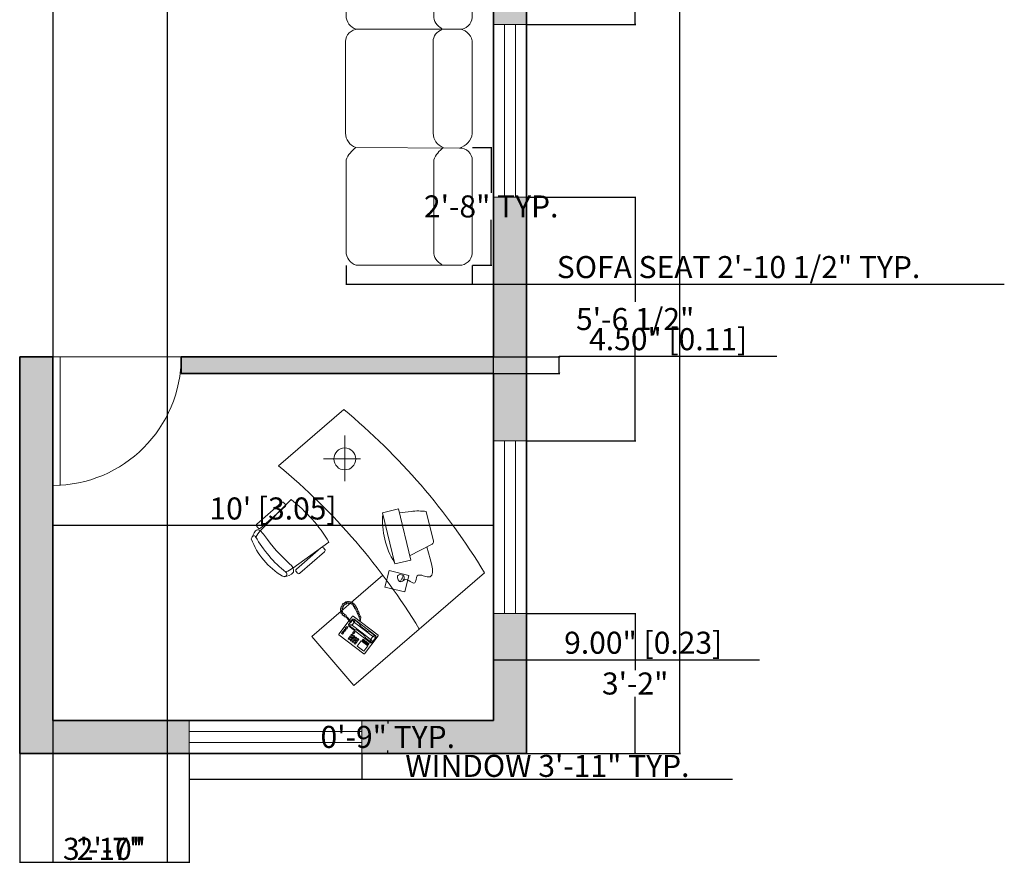
# Model space of a CAD drawing. Units: inches. Extents: x 2322 to 2932, y 142 to 762.
# Tile 2 of 7: x 2664 to 2932, y 146 to 376. Entities that reach past the tile are written whole.
import ezdxf

# ---------------------------------------------------------------- set-up
doc = ezdxf.new("R2010")
doc.units = ezdxf.units.IN
doc.header["$MEASUREMENT"] = 0
for name, color, linetype, lineweight in [('A-ANNO-DIMS', 2, 'Continuous', 18), ('A-DOOR', 3, 'Continuous', 18), ('A-EQPM', 8, 'Continuous', 15), ('A-GLAZ', 4, 'Continuous', 18), ('A-WALL', 7, 'Continuous', 35)]:
    doc.layers.add(name, color=color, linetype=linetype, lineweight=lineweight)
doc.layers.add('A-WALL-PATT', color=40, linetype='Continuous', lineweight=13, true_color=0xf8d731)
doc.layers.add('Furniture', color=7, linetype='Continuous', lineweight=15, true_color=0xffffff)
doc.styles.get("Standard").update_dxf_attribs({"font": 'italic8.shx'})
doc.dimstyles.get("Standard").update_dxf_attribs({"dimtxt": 6, "dimasz": 0.15, "dimexe": 0.18, "dimexo": 0.0625, "dimgap": 0.09, "dimtad": 1, "dimtih": 1, "dimtoh": 1, "dimzin": 0, "dimdsep": 46, "dimlunit": 3, "dimtxsty": 'Standard', "dimblk": 'CLOSEDBLANK', "dimcen": 0.09, "dimclrd": 3, "dimclre": 1, "dimclrt": 6, "dimadec": 0, "dimazin": 0, "dimtfac": 1, "dimtofl": 0, "dimtmove": 0, "dimatfit": 3, "dimldrblk": 'DOT', "dimfxl": 1, "dimtolj": 1, "dimtzin": 0, "dimarcsym": 0})

# ---------------------------------------------------------------- blocks, each defined once
blk = doc.blocks.new('_ClosedBlank')
at = {"color": 0, "linetype": 'ByBlock', "lineweight": -2}
for p, q in [((-1, 0.2), (0, 0)), ((-1, 0.2), (-1, -0.2)), ((0, 0), (-1, -0.2))]:
    blk.add_line(p, q, dxfattribs=at)
blk = doc.blocks.new('*D3')
at = {"layer": 'A-ANNO-DIMS', "color": 0, "lineweight": -2, "transparency": 16777216}
for p, q in [((2802.13, 718.82), (2844.02, 718.82)), ((2843.84, 718.67), (2843.84, 451.98)), ((2843.84, 175.97), (2843.84, 442.66)), ((2802.13, 175.82), (2844.02, 175.82))]:
    blk.add_line(p, q, dxfattribs=at)
at = {"layer": 'Defpoints', "color": 0, "transparency": 16777216}
for p in [(2802.06, 718.82), (2802.06, 175.82), (2843.84, 175.82)]:
    blk.add_point(p, dxfattribs=at)
at = {"layer": 'A-ANNO-DIMS', "color": 0, "lineweight": -2, "transparency": 16777216, "xscale": 0.15, "yscale": 0.15, "zscale": 0.15}
for p, rotation in [((2843.84, 718.82), 90), ((2843.84, 175.82), 270)]:
    blk.add_blockref('_ClosedBlank', p, dxfattribs=dict(at, rotation=rotation))
at = {"layer": 'A-ANNO-DIMS', "color": 0, "transparency": 16777216, "insert": (2843.84, 447.32), "char_height": 6, "attachment_point": 5}
blk.add_mtext('\\A1;45\'-3.00" [13.79]', dxfattribs=at)
blk = doc.blocks.new('_Dot')
at = {"color": 0, "linetype": 'ByBlock', "lineweight": -2}
blk.add_line((-0.5, 0), (-1, 0), dxfattribs=at)
at = {"color": 0, "linetype": 'ByBlock', "const_width": 0.5}
blk.add_lwpolyline([(-0.25, 0, 1), (0.25, 0, 1)], format="xyb", close=True, dxfattribs=at)
blk = doc.blocks.new('*D4')
at = {"layer": 'A-ANNO-DIMS', "color": 0, "lineweight": -2, "transparency": 16777216}
for p, q in [((2673.06, 234.35), (2673.06, 238.01)), ((2792.91, 237.83), (2673.21, 237.83)), ((2793.06, 237.77), (2793.06, 237.65))]:
    blk.add_line(p, q, dxfattribs=at)
at = {"layer": 'Defpoints', "color": 0, "transparency": 16777216}
for p in [(2673.06, 237.83), (2793.06, 237.83), (2673.06, 234.29)]:
    blk.add_point(p, dxfattribs=at)
at = {"layer": 'A-ANNO-DIMS', "color": 0, "lineweight": -2, "transparency": 16777216, "xscale": 0.15, "yscale": 0.15, "zscale": 0.15, "rotation": 180}
blk.add_blockref('_ClosedBlank', (2673.06, 237.83), dxfattribs=at)
at = {"layer": 'A-ANNO-DIMS', "color": 0, "lineweight": -2, "transparency": 16777216, "xscale": 0.15, "yscale": 0.15, "zscale": 0.15}
blk.add_blockref('_ClosedBlank', (2793.06, 237.83), dxfattribs=at)
at = {"layer": 'A-ANNO-DIMS', "color": 0, "transparency": 16777216, "insert": (2733.06, 242.49), "char_height": 6, "attachment_point": 5}
blk.add_mtext("\\A1;10' [3.05]", dxfattribs=at)
blk = doc.blocks.new('*D5')
at = {"layer": 'A-ANNO-DIMS', "color": 0, "lineweight": -2, "transparency": 16777216}
for p, q in [((2793.06, 307.6), (2793.06, 201.1)), ((2802.06, 307.6), (2802.06, 201.1)), ((2793.21, 201.28), (2801.91, 201.28)), ((2802.06, 201.28), (2865.54, 201.28))]:
    blk.add_line(p, q, dxfattribs=at)
at = {"layer": 'Defpoints', "color": 0, "transparency": 16777216}
for p in [(2793.06, 307.66), (2802.06, 307.66), (2802.06, 201.28)]:
    blk.add_point(p, dxfattribs=at)
at = {"layer": 'A-ANNO-DIMS', "color": 0, "lineweight": -2, "transparency": 16777216, "xscale": 0.15, "yscale": 0.15, "zscale": 0.15, "rotation": 180}
blk.add_blockref('_ClosedBlank', (2793.06, 201.28), dxfattribs=at)
at = {"layer": 'A-ANNO-DIMS', "color": 0, "lineweight": -2, "transparency": 16777216, "xscale": 0.15, "yscale": 0.15, "zscale": 0.15}
blk.add_blockref('_ClosedBlank', (2802.06, 201.28), dxfattribs=at)
at = {"layer": 'A-ANNO-DIMS', "color": 0, "transparency": 16777216, "insert": (2833.88, 205.95), "char_height": 6, "attachment_point": 5}
blk.add_mtext('\\A1;9.00" [0.23]', dxfattribs=at)
blk = doc.blocks.new('*D6')
at = {"layer": 'A-ANNO-DIMS', "color": 0, "lineweight": -2, "transparency": 16777216}
for p, q in [((2743.62, 283.76), (2811.19, 283.76)), ((2811.01, 283.76), (2811.01, 283.91)), ((2811.01, 283.91), (2870.24, 283.91)), ((2811.01, 279.41), (2811.01, 283.61)), ((2743.62, 279.26), (2811.19, 279.26))]:
    blk.add_line(p, q, dxfattribs=at)
at = {"layer": 'Defpoints', "color": 0, "transparency": 16777216}
for p in [(2743.55, 283.76), (2811.01, 283.76), (2743.55, 279.26)]:
    blk.add_point(p, dxfattribs=at)
at = {"layer": 'A-ANNO-DIMS', "color": 0, "lineweight": -2, "transparency": 16777216, "xscale": 0.15, "yscale": 0.15, "zscale": 0.15}
for p, rotation in [((2811.01, 283.76), 90), ((2811.01, 279.26), 270)]:
    blk.add_blockref('_ClosedBlank', p, dxfattribs=dict(at, rotation=rotation))
at = {"layer": 'A-ANNO-DIMS', "color": 0, "transparency": 16777216, "insert": (2840.67, 288.57), "char_height": 6, "attachment_point": 5}
blk.add_mtext('\\A1;4.50" [0.11]', dxfattribs=at)
blk = doc.blocks.new('DOOR-SWING-35')
for p, q in [((0, 35), (0, 0)), ((2, 35), (2, 0)), ((0, 0), (35, 0))]:
    blk.add_line(p, q)
blk.add_arc((0, 0), 35, 0, 90)
blk = doc.blocks.new('WINDOW-47X9')
for p, q in [((47, 9), (0, 9)), ((0, 9), (0, 0)), ((47, 0), (47, 9)), ((0, 6), (47, 6)), ((0, 3), (47, 3)), ((0, 0), (47, 0))]:
    blk.add_line(p, q)
blk = doc.blocks.new('SECTIONAL-SEAT')
for p, q in [((30.86, 31.9), (2.62, 32.04)), ((0, 28.69), (0, 3.79)), ((23.85, 28.69), (23.85, 3.79)), ((34.36, 3.2), (34.36, 28.55)), ((2.77, 0), (30.86, 0))]:
    blk.add_line(p, q)
for centre, radius, start, end in [((7.53, 25.51), 8.17, 126.8838, 157.0502), ((31.38, 25.51), 8.17, 126.8838, 157.0502), ((31, 28.55), 3.35, 0, 92.4088), ((3.98, 3.79), 3.98, 180, 252.2888), ((27.83, 3.79), 3.98, 180, 244.0743), ((30.86, 3.51), 3.51, 270, 355.0498)]:
    blk.add_arc(centre, radius, start, end)
blk = doc.blocks.new('*D28')
at = {"layer": 'A-ANNO-DIMS', "color": 1, "lineweight": -2, "transparency": 16777216}
for p, q in [((2710.26, 175.76), (2710.26, 168.59)), ((2757.26, 175.76), (2757.26, 168.59))]:
    blk.add_line(p, q, dxfattribs=at)
at = {"layer": 'A-ANNO-DIMS', "color": 3, "lineweight": -2, "transparency": 16777216}
for p, q in [((2710.41, 168.77), (2757.11, 168.77)), ((2757.26, 168.77), (2858.16, 168.77))]:
    blk.add_line(p, q, dxfattribs=at)
at = {"layer": 'Defpoints', "color": 0, "transparency": 16777216}
for p in [(2710.26, 175.82), (2757.26, 175.82), (2757.26, 168.77)]:
    blk.add_point(p, dxfattribs=at)
at = {"layer": 'A-ANNO-DIMS', "color": 3, "lineweight": -2, "transparency": 16777216, "xscale": 0.15, "yscale": 0.15, "zscale": 0.15, "rotation": 180}
blk.add_blockref('_ClosedBlank', (2710.26, 168.77), dxfattribs=at)
at = {"layer": 'A-ANNO-DIMS', "color": 3, "lineweight": -2, "transparency": 16777216, "xscale": 0.15, "yscale": 0.15, "zscale": 0.15}
blk.add_blockref('_ClosedBlank', (2757.26, 168.77), dxfattribs=at)
at = {"layer": 'A-ANNO-DIMS', "color": 6, "transparency": 16777216, "insert": (2807.78, 172.43), "char_height": 6, "attachment_point": 5}
blk.add_mtext('\\A1;WINDOW 3\'-11" TYP.', dxfattribs=at)
blk = doc.blocks.new('*D29')
at = {"layer": 'A-ANNO-DIMS', "color": 1, "lineweight": -2, "transparency": 16777216}
for p, q in [((2757.32, 184.82), (2764.49, 184.82)), ((2757.32, 175.82), (2764.49, 175.82))]:
    blk.add_line(p, q, dxfattribs=at)
at = {"layer": 'A-ANNO-DIMS', "color": 3, "lineweight": -2, "transparency": 16777216}
for p, q in [((2764.31, 184.67), (2764.31, 183.98)), ((2764.31, 175.97), (2764.31, 176.66))]:
    blk.add_line(p, q, dxfattribs=at)
at = {"layer": 'Defpoints', "color": 0, "transparency": 16777216}
for p in [(2757.26, 184.82), (2764.31, 184.82), (2757.26, 175.82)]:
    blk.add_point(p, dxfattribs=at)
at = {"layer": 'A-ANNO-DIMS', "color": 3, "lineweight": -2, "transparency": 16777216, "xscale": 0.15, "yscale": 0.15, "zscale": 0.15}
for p, rotation in [((2764.31, 184.82), 90), ((2764.31, 175.82), 270)]:
    blk.add_blockref('_ClosedBlank', p, dxfattribs=dict(at, rotation=rotation))
at = {"layer": 'A-ANNO-DIMS', "color": 6, "transparency": 16777216, "insert": (2764.31, 180.32), "char_height": 6, "attachment_point": 5}
blk.add_mtext('\\A1;0\'-9" TYP.', dxfattribs=at)
blk = doc.blocks.new('*D40')
at = {"layer": 'A-ANNO-DIMS', "color": 1, "lineweight": -2, "transparency": 16777216}
for p, q in [((2752.97, 308.61), (2752.97, 303.34)), ((2787.33, 308.61), (2787.33, 303.34))]:
    blk.add_line(p, q, dxfattribs=at)
at = {"layer": 'A-ANNO-DIMS', "color": 3, "lineweight": -2, "transparency": 16777216}
for p, q in [((2753.12, 303.52), (2787.18, 303.52)), ((2787.33, 303.52), (2932.23, 303.52))]:
    blk.add_line(p, q, dxfattribs=at)
at = {"layer": 'Defpoints', "color": 0, "transparency": 16777216}
for p in [(2752.97, 308.68), (2787.33, 308.68), (2787.33, 303.52)]:
    blk.add_point(p, dxfattribs=at)
at = {"layer": 'A-ANNO-DIMS', "color": 3, "lineweight": -2, "transparency": 16777216, "xscale": 0.15, "yscale": 0.15, "zscale": 0.15, "rotation": 180}
blk.add_blockref('_ClosedBlank', (2752.97, 303.52), dxfattribs=at)
at = {"layer": 'A-ANNO-DIMS', "color": 3, "lineweight": -2, "transparency": 16777216, "xscale": 0.15, "yscale": 0.15, "zscale": 0.15}
blk.add_blockref('_ClosedBlank', (2787.33, 303.52), dxfattribs=at)
at = {"layer": 'A-ANNO-DIMS', "color": 6, "transparency": 16777216, "insert": (2859.85, 308.19), "char_height": 6, "attachment_point": 5}
blk.add_mtext('\\A1;SOFA SEAT 2\'-10 1/2" TYP.', dxfattribs=at)
blk = doc.blocks.new('*D41')
at = {"layer": 'A-ANNO-DIMS', "color": 1, "lineweight": -2, "transparency": 16777216}
for p, q in [((2787.39, 340.72), (2792.66, 340.72)), ((2787.39, 308.68), (2792.66, 308.68))]:
    blk.add_line(p, q, dxfattribs=at)
at = {"layer": 'A-ANNO-DIMS', "color": 3, "lineweight": -2, "transparency": 16777216}
for p, q in [((2792.48, 340.57), (2792.48, 328.36)), ((2792.48, 308.83), (2792.48, 321.04))]:
    blk.add_line(p, q, dxfattribs=at)
at = {"layer": 'Defpoints', "color": 0, "transparency": 16777216}
for p in [(2787.33, 340.72), (2792.48, 340.72), (2787.33, 308.68)]:
    blk.add_point(p, dxfattribs=at)
at = {"layer": 'A-ANNO-DIMS', "color": 3, "lineweight": -2, "transparency": 16777216, "xscale": 0.15, "yscale": 0.15, "zscale": 0.15}
for p, rotation in [((2792.48, 340.72), 90), ((2792.48, 308.68), 270)]:
    blk.add_blockref('_ClosedBlank', p, dxfattribs=dict(at, rotation=rotation))
at = {"layer": 'A-ANNO-DIMS', "color": 6, "transparency": 16777216, "insert": (2792.48, 324.7), "char_height": 6, "attachment_point": 5}
blk.add_mtext('\\A1;2\'-8" TYP.', dxfattribs=at)
blk = doc.blocks.new('*D54')
at = {"layer": 'A-ANNO-DIMS', "color": 1, "lineweight": -2, "transparency": 16777216}
for p, q in [((2673.06, 709.76), (2673.06, 146.01)), ((2704.23, 709.76), (2704.23, 146.01))]:
    blk.add_line(p, q, dxfattribs=at)
at = {"layer": 'A-ANNO-DIMS', "color": 3, "lineweight": -2, "transparency": 16777216}
blk.add_line((2673.21, 146.19), (2704.08, 146.19), dxfattribs=at)
at = {"layer": 'Defpoints', "color": 0, "transparency": 16777216}
for p in [(2673.06, 709.82), (2704.23, 709.82), (2704.23, 146.19)]:
    blk.add_point(p, dxfattribs=at)
at = {"layer": 'A-ANNO-DIMS', "color": 3, "lineweight": -2, "transparency": 16777216, "xscale": 0.15, "yscale": 0.15, "zscale": 0.15, "rotation": 180}
blk.add_blockref('_ClosedBlank', (2673.06, 146.19), dxfattribs=at)
at = {"layer": 'A-ANNO-DIMS', "color": 3, "lineweight": -2, "transparency": 16777216, "xscale": 0.15, "yscale": 0.15, "zscale": 0.15}
blk.add_blockref('_ClosedBlank', (2704.23, 146.19), dxfattribs=at)
at = {"layer": 'A-ANNO-DIMS', "color": 6, "transparency": 16777216, "insert": (2688.65, 149.85), "char_height": 6, "attachment_point": 5}
blk.add_mtext('\\A1;2\'-7"', dxfattribs=at)
blk = doc.blocks.new('*D61')
at = {"layer": 'A-ANNO-DIMS', "color": 1, "lineweight": -2, "transparency": 16777216}
for p, q in [((2802.13, 213.88), (2831.87, 213.88)), ((2802.13, 175.82), (2831.87, 175.82))]:
    blk.add_line(p, q, dxfattribs=at)
at = {"layer": 'A-ANNO-DIMS', "color": 3, "lineweight": -2, "transparency": 16777216}
for p, q in [((2831.69, 213.73), (2831.69, 198.51)), ((2831.69, 175.97), (2831.69, 191.19))]:
    blk.add_line(p, q, dxfattribs=at)
at = {"layer": 'Defpoints', "color": 0, "transparency": 16777216}
for p in [(2802.06, 213.88), (2831.69, 213.88), (2802.06, 175.82)]:
    blk.add_point(p, dxfattribs=at)
at = {"layer": 'A-ANNO-DIMS', "color": 3, "lineweight": -2, "transparency": 16777216, "xscale": 0.15, "yscale": 0.15, "zscale": 0.15}
for p, rotation in [((2831.69, 213.88), 90), ((2831.69, 175.82), 270)]:
    blk.add_blockref('_ClosedBlank', p, dxfattribs=dict(at, rotation=rotation))
at = {"layer": 'A-ANNO-DIMS', "color": 6, "transparency": 16777216, "insert": (2831.69, 194.85), "char_height": 6, "attachment_point": 5}
blk.add_mtext('\\A1;3\'-2"', dxfattribs=at)
blk = doc.blocks.new('*D62')
at = {"layer": 'A-ANNO-DIMS', "color": 1, "lineweight": -2, "transparency": 16777216}
for p, q in [((2802.13, 327.22), (2831.87, 327.22)), ((2802.13, 260.88), (2831.87, 260.88))]:
    blk.add_line(p, q, dxfattribs=at)
at = {"layer": 'A-ANNO-DIMS', "color": 3, "lineweight": -2, "transparency": 16777216}
for p, q in [((2831.69, 327.07), (2831.69, 298.71)), ((2831.69, 261.03), (2831.69, 289.39))]:
    blk.add_line(p, q, dxfattribs=at)
at = {"layer": 'Defpoints', "color": 0, "transparency": 16777216}
for p in [(2802.06, 327.22), (2831.69, 327.22), (2802.06, 260.88)]:
    blk.add_point(p, dxfattribs=at)
at = {"layer": 'A-ANNO-DIMS', "color": 3, "lineweight": -2, "transparency": 16777216, "xscale": 0.15, "yscale": 0.15, "zscale": 0.15}
for p, rotation in [((2831.69, 327.22), 90), ((2831.69, 260.88), 270)]:
    blk.add_blockref('_ClosedBlank', p, dxfattribs=dict(at, rotation=rotation))
at = {"layer": 'A-ANNO-DIMS', "color": 6, "transparency": 16777216, "insert": (2831.69, 294.05), "char_height": 6, "attachment_point": 5}
blk.add_mtext('\\A1;5\'-6 1/2"', dxfattribs=at)
blk = doc.blocks.new('*D63')
at = {"layer": 'A-ANNO-DIMS', "color": 1, "lineweight": -2, "transparency": 16777216}
for p, q in [((2802.13, 431.57), (2831.87, 431.57)), ((2802.13, 374.22), (2831.87, 374.22))]:
    blk.add_line(p, q, dxfattribs=at)
at = {"layer": 'A-ANNO-DIMS', "color": 3, "lineweight": -2, "transparency": 16777216}
for p, q in [((2831.69, 431.42), (2831.69, 407.55)), ((2831.69, 374.37), (2831.69, 398.23))]:
    blk.add_line(p, q, dxfattribs=at)
at = {"layer": 'Defpoints', "color": 0, "transparency": 16777216}
for p in [(2802.06, 431.57), (2831.69, 431.57), (2802.06, 374.22)]:
    blk.add_point(p, dxfattribs=at)
at = {"layer": 'A-ANNO-DIMS', "color": 3, "lineweight": -2, "transparency": 16777216, "xscale": 0.15, "yscale": 0.15, "zscale": 0.15}
for p, rotation in [((2831.69, 431.57), 90), ((2831.69, 374.22), 270)]:
    blk.add_blockref('_ClosedBlank', p, dxfattribs=dict(at, rotation=rotation))
at = {"layer": 'A-ANNO-DIMS', "color": 6, "transparency": 16777216, "insert": (2831.69, 402.89), "char_height": 6, "attachment_point": 5}
blk.add_mtext('\\A1;4\'-9 1/2"', dxfattribs=at)
blk = doc.blocks.new('*D65')
at = {"layer": 'A-ANNO-DIMS', "color": 1, "lineweight": -2, "transparency": 16777216}
for p, q in [((2664.06, 175.76), (2664.06, 146.01)), ((2710.26, 175.76), (2710.26, 146.01))]:
    blk.add_line(p, q, dxfattribs=at)
at = {"layer": 'A-ANNO-DIMS', "color": 3, "lineweight": -2, "transparency": 16777216}
blk.add_line((2664.21, 146.19), (2710.11, 146.19), dxfattribs=at)
at = {"layer": 'Defpoints', "color": 0, "transparency": 16777216}
for p in [(2664.06, 175.82), (2710.26, 175.82), (2710.26, 146.19)]:
    blk.add_point(p, dxfattribs=at)
at = {"layer": 'A-ANNO-DIMS', "color": 3, "lineweight": -2, "transparency": 16777216, "xscale": 0.15, "yscale": 0.15, "zscale": 0.15, "rotation": 180}
blk.add_blockref('_ClosedBlank', (2664.06, 146.19), dxfattribs=at)
at = {"layer": 'A-ANNO-DIMS', "color": 3, "lineweight": -2, "transparency": 16777216, "xscale": 0.15, "yscale": 0.15, "zscale": 0.15}
blk.add_blockref('_ClosedBlank', (2710.26, 146.19), dxfattribs=at)
at = {"layer": 'A-ANNO-DIMS', "color": 6, "transparency": 16777216, "insert": (2687.16, 149.85), "char_height": 6, "attachment_point": 5}
blk.add_mtext('\\A1;3\'-10"', dxfattribs=at)

msp = doc.modelspace()

# ---------------------------------------------------------------- hatches: boundary and pattern name
at = {"layer": 'A-WALL-PATT'}
h = msp.add_hatch(color=256, dxfattribs=at)
h.dxf.hatch_style = 1
h.paths.add_polyline_path([(2559.693, 283.756), (2439.065, 283.756), (2439.065, 295.453), (2430.065, 295.453), (2430.065, 274.756), (2559.693, 274.756)])
h.paths.add_polyline_path([(2802.065, 431.568), (2793.065, 431.568), (2793.065, 374.218), (2802.065, 374.218)])
h.paths.add_polyline_path([(2802.065, 327.218), (2793.065, 327.218), (2793.065, 283.756), (2708.065, 283.756), (2708.065, 279.256), (2793.065, 279.256), (2793.065, 260.879), (2802.065, 260.879)])
h.paths.add_polyline_path([(2673.065, 283.756), (2664.065, 283.756), (2664.065, 175.819), (2710.255, 175.819), (2710.255, 184.819), (2673.065, 184.819)])
h.paths.add_polyline_path([(2802.065, 213.879), (2793.065, 213.879), (2793.065, 184.819), (2757.255, 184.819), (2757.255, 175.819), (2802.065, 175.819)])

# ---------------------------------------------------------------- linework, layer by layer
at = {"layer": 'A-EQPM'}
for p, q in [((2767.2, 242.392), (2762.863, 241.346)), ((2770.565, 228.443), (2767.2, 242.392)), ((2767.439, 241.306), (2770.668, 241.706)), ((2776.743, 233.57), (2774.796, 241.654)), ((2762.863, 241.346), (2766.228, 227.397)), ((2770.276, 229.637), (2776.445, 232.795)), ((2766.228, 227.397), (2770.565, 228.443)), ((2763.556, 221.103), (2764.685, 225.623)), ((2764.685, 225.623), (2770.048, 224.284)), ((2767.727, 222.541), (2768.488, 224.187)), ((2768.767, 223.098), (2768.158, 223.402)), ((2770.048, 224.284), (2768.919, 219.764)), ((2768.919, 219.764), (2763.556, 221.103)), ((2751.408, 214.719), (2751.752, 214.818)), ((2751.473, 214.432), (2751.408, 214.719)), ((2751.453, 214.984), (2751.477, 215.264)), ((2751.752, 214.818), (2751.453, 214.984)), ((2751.477, 215.264), (2751.859, 215.351)), ((2751.507, 215.573), (2751.607, 215.827)), ((2751.859, 215.351), (2751.507, 215.573)), ((2751.607, 215.827), (2751.975, 215.752)), ((2751.797, 216.076), (2751.907, 216.261)), ((2751.975, 215.752), (2751.797, 216.076)), ((2751.907, 216.261), (2752.249, 216.11)), ((2752.046, 215.555), (2751.923, 214.814)), ((2751.923, 214.814), (2752.112, 214.071)), ((2752.013, 216.463), (2752.208, 216.614)), ((2752.249, 216.11), (2752.013, 216.463)), ((2752.453, 216.191), (2752.046, 215.555)), ((2752.208, 216.614), (2752.484, 216.419)), ((2753.143, 216.579), (2752.453, 216.191)), ((2752.46, 216.8), (2752.661, 216.899)), ((2752.484, 216.419), (2752.46, 216.8)), ((2752.661, 216.899), (2752.938, 216.641)), ((2752.838, 217.048), (2753.099, 217.101)), ((2752.938, 216.641), (2752.838, 217.048)), ((2753.099, 217.101), (2753.277, 216.776)), ((2753.906, 216.69), (2753.143, 216.579)), ((2753.277, 216.776), (2753.37, 217.146)), ((2753.37, 217.146), (2753.589, 217.184)), ((2753.589, 217.184), (2753.751, 216.839)), ((2753.751, 216.839), (2753.882, 217.197)), ((2753.882, 217.197), (2754.142, 217.124)), ((2754.76, 216.259), (2753.906, 216.69)), ((2754.142, 217.124), (2754.229, 216.68)), ((2754.229, 216.68), (2754.455, 216.996)), ((2754.455, 216.996), (2754.685, 216.884)), ((2754.685, 216.884), (2754.636, 216.511)), ((2754.636, 216.511), (2754.962, 216.751)), ((2755.446, 215.216), (2754.76, 216.259)), ((2754.962, 216.751), (2755.173, 216.511)), ((2755.173, 216.511), (2754.968, 216.242)), ((2754.968, 216.242), (2755.327, 216.3)), ((2755.503, 216.055), (2755.25, 215.744)), ((2755.25, 215.744), (2755.58, 215.949)), ((2755.327, 216.3), (2755.503, 216.055)), ((2755.781, 214.456), (2755.446, 215.216)), ((2755.81, 215.631), (2755.552, 215.355)), ((2755.552, 215.355), (2755.978, 215.314)), ((2755.58, 215.949), (2755.81, 215.631)), ((2756.054, 215.083), (2755.762, 214.864)), ((2755.762, 214.864), (2756.145, 214.809)), ((2756.271, 214.539), (2755.976, 214.339)), ((2755.978, 215.314), (2756.054, 215.083)), ((2756.145, 214.809), (2756.271, 214.539)), ((2753.786, 211.958), (2750.971, 208.269)), ((2751.859, 214.359), (2751.473, 214.432)), ((2751.571, 214.105), (2751.859, 214.359)), ((2751.702, 213.801), (2751.571, 214.105)), ((2752.134, 213.913), (2751.702, 213.801)), ((2751.92, 213.571), (2752.134, 213.913)), ((2752.174, 213.346), (2751.92, 213.571)), ((2752.112, 214.071), (2752.702, 213.542)), ((2752.557, 213.495), (2752.174, 213.346)), ((2752.386, 213.168), (2752.557, 213.495)), ((2752.64, 213.006), (2752.386, 213.168)), ((2752.834, 213.032), (2752.64, 213.006)), ((2752.702, 213.542), (2752.962, 213.407)), ((2752.871, 212.956), (2752.834, 213.032)), ((2753.138, 212.769), (2752.871, 212.956)), ((2752.962, 213.407), (2752.955, 213.129)), ((2752.955, 213.129), (2753.222, 212.941)), ((2753.515, 212.292), (2753.138, 212.769)), ((2753.222, 212.941), (2753.438, 212.728)), ((2753.438, 212.728), (2753.815, 212.251)), ((2753.922, 211.792), (2753.515, 212.292)), ((2753.815, 212.251), (2754.081, 211.938)), ((2754.727, 213.192), (2753.918, 212.131)), ((2754.081, 211.938), (2754.454, 211.609)), ((2754.708, 212.35), (2754.268, 211.773)), ((2754.315, 211.732), (2754.682, 212.214)), ((2754.682, 212.214), (2754.931, 212.335)), ((2755.134, 211.479), (2754.682, 212.214)), ((2755.191, 212.37), (2754.708, 212.35)), ((2754.901, 213.215), (2754.727, 213.192)), ((2761.694, 208.032), (2754.901, 213.215)), ((2754.931, 212.335), (2755.165, 212.234)), ((2755.165, 212.234), (2755.27, 211.453)), ((2755.165, 212.234), (2756.494, 211.22)), ((2761.098, 207.864), (2755.191, 212.37)), ((2755.884, 214.425), (2755.781, 214.456)), ((2755.85, 214.34), (2755.884, 214.425)), ((2756.099, 213.819), (2755.85, 214.34)), ((2755.976, 214.339), (2756.342, 214.343)), ((2756.395, 213.089), (2756.099, 213.819)), ((2756.485, 214.076), (2756.16, 213.898)), ((2756.16, 213.898), (2756.549, 213.933)), ((2756.648, 213.731), (2756.338, 213.511)), ((2756.338, 213.511), (2756.748, 213.45)), ((2756.342, 214.343), (2756.485, 214.076)), ((2756.557, 212.682), (2756.395, 213.089)), ((2756.549, 213.933), (2756.648, 213.731)), ((2756.748, 212.725), (2756.557, 212.682)), ((2756.837, 213.256), (2756.56, 213.058)), ((2756.56, 213.058), (2756.941, 213.019)), ((2756.575, 211.938), (2756.673, 212.152)), ((2756.672, 212.626), (2756.748, 212.725)), ((2756.686, 212.52), (2756.672, 212.626)), ((2756.673, 212.152), (2756.677, 212.322)), ((2756.677, 212.322), (2756.686, 212.52)), ((2756.901, 212.12), (2756.722, 211.825)), ((2756.748, 213.45), (2756.837, 213.256)), ((2756.966, 212.764), (2756.839, 212.577)), ((2756.839, 212.577), (2756.922, 212.293)), ((2756.922, 212.293), (2756.901, 212.12)), ((2756.941, 213.019), (2757.02, 212.896)), ((2757.02, 212.896), (2756.966, 212.764)), ((2752.217, 209.187), (2752.593, 209.68)), ((2752.513, 208.962), (2752.217, 209.187)), ((2752.888, 209.454), (2752.513, 208.962)), ((2752.593, 209.68), (2752.888, 209.454)), ((2752.743, 209.876), (2753.119, 210.369)), ((2753.039, 209.651), (2752.743, 209.876)), ((2753.414, 210.143), (2753.039, 209.651)), ((2753.119, 210.369), (2753.414, 210.143)), ((2754.147, 211.614), (2753.619, 210.922)), ((2753.619, 210.922), (2753.677, 210.488)), ((2753.677, 210.488), (2759.634, 205.944)), ((2753.781, 211.032), (2753.729, 210.76)), ((2753.729, 210.76), (2753.888, 210.561)), ((2753.781, 211.032), (2754.196, 211.576)), ((2754.608, 210.79), (2753.781, 211.032)), ((2753.888, 210.561), (2754.669, 210.666)), ((2753.888, 210.561), (2755.217, 209.547)), ((2754.341, 211.461), (2753.922, 211.792)), ((2754.454, 211.609), (2754.341, 211.461)), ((2755.134, 211.479), (2754.608, 210.79)), ((2754.669, 210.666), (2754.608, 210.79)), ((2757.328, 208.638), (2754.669, 210.666)), ((2755.27, 211.453), (2755.134, 211.479)), ((2755.217, 209.547), (2755.539, 209.457)), ((2757.929, 209.425), (2755.27, 211.453)), ((2755.539, 209.457), (2755.897, 209.417)), ((2755.897, 209.417), (2756.28, 209.203)), ((2756.28, 209.203), (2757.215, 208.49)), ((2756.494, 211.22), (2756.665, 210.934)), ((2756.665, 210.934), (2756.799, 210.599)), ((2756.799, 210.599), (2757.106, 210.286)), ((2757.106, 210.286), (2758.041, 209.573)), ((2757.929, 209.425), (2760.144, 207.735)), ((2758.533, 209.197), (2758.041, 209.573)), ((2758.916, 208.984), (2758.533, 209.197)), ((2750.971, 208.269), (2750.995, 208.095)), ((2750.995, 208.095), (2757.788, 202.912)), ((2751.692, 208.498), (2752.067, 208.99)), ((2751.987, 208.273), (2751.692, 208.498)), ((2752.363, 208.765), (2751.987, 208.273)), ((2752.067, 208.99), (2752.363, 208.765)), ((2753.75, 207.317), (2753.525, 207.022)), ((2753.525, 207.022), (2753.82, 206.796)), ((2754.045, 207.092), (2753.75, 207.317)), ((2753.82, 206.796), (2754.045, 207.092)), ((2754.126, 207.809), (2753.9, 207.514)), ((2753.9, 207.514), (2754.196, 207.289)), ((2754.292, 206.904), (2754.066, 206.609)), ((2754.066, 206.609), (2754.362, 206.383)), ((2754.421, 207.584), (2754.126, 207.809)), ((2754.196, 207.289), (2754.421, 207.584)), ((2754.501, 208.302), (2754.276, 208.006)), ((2754.276, 208.006), (2754.571, 207.781)), ((2754.587, 206.679), (2754.292, 206.904)), ((2754.362, 206.383), (2754.587, 206.679)), ((2754.667, 207.396), (2754.442, 207.101)), ((2754.442, 207.101), (2754.737, 206.875)), ((2754.797, 208.076), (2754.501, 208.302)), ((2754.571, 207.781), (2754.797, 208.076)), ((2754.833, 206.491), (2754.608, 206.195)), ((2754.963, 207.171), (2754.667, 207.396)), ((2755.027, 208.991), (2754.727, 208.597)), ((2754.727, 208.597), (2755.022, 208.372)), ((2754.737, 206.875), (2754.963, 207.171)), ((2755.043, 207.888), (2754.817, 207.593)), ((2754.817, 207.593), (2755.113, 207.368)), ((2755.128, 206.265), (2754.833, 206.491)), ((2755.209, 206.983), (2754.983, 206.688)), ((2754.983, 206.688), (2755.279, 206.462)), ((2755.022, 208.372), (2755.322, 208.765)), ((2755.322, 208.765), (2755.027, 208.991)), ((2755.338, 207.663), (2755.043, 207.888)), ((2755.113, 207.368), (2755.338, 207.663)), ((2755.504, 206.758), (2755.209, 206.983)), ((2755.279, 206.462), (2755.504, 206.758)), ((2755.584, 207.475), (2755.359, 207.18)), ((2755.359, 207.18), (2755.654, 206.955)), ((2755.75, 206.57), (2755.525, 206.275)), ((2755.88, 207.25), (2755.584, 207.475)), ((2755.654, 206.955), (2755.88, 207.25)), ((2756.046, 206.345), (2755.75, 206.57)), ((2756.126, 207.062), (2755.9, 206.767)), ((2755.9, 206.767), (2756.196, 206.542)), ((2756.421, 206.837), (2756.126, 207.062)), ((2756.196, 206.542), (2756.421, 206.837)), ((2757.707, 208.114), (2757.215, 208.49)), ((2757.298, 206.557), (2757.599, 206.951)), ((2757.446, 206.445), (2757.298, 206.557)), ((2757.328, 208.638), (2759.543, 206.947)), ((2757.746, 206.838), (2757.446, 206.445)), ((2757.594, 206.332), (2757.894, 206.726)), ((2757.599, 206.951), (2757.746, 206.838)), ((2758.014, 207.802), (2757.707, 208.114)), ((2758.042, 206.613), (2757.741, 206.219)), ((2757.889, 206.107), (2758.189, 206.5)), ((2757.894, 206.726), (2758.042, 206.613)), ((2757.962, 202.936), (2761.718, 207.858)), ((2758.148, 207.467), (2758.014, 207.802)), ((2758.319, 207.18), (2758.148, 207.467)), ((2758.189, 206.5), (2758.337, 206.388)), ((2759.648, 206.166), (2758.319, 207.18)), ((2759.274, 208.944), (2758.916, 208.984)), ((2759.596, 208.854), (2759.274, 208.944)), ((2759.543, 206.947), (2759.679, 206.922)), ((2759.648, 206.166), (2759.543, 206.947)), ((2760.925, 207.84), (2759.596, 208.854)), ((2760.205, 207.611), (2759.679, 206.922)), ((2759.679, 206.922), (2760.131, 206.187)), ((2760.03, 205.953), (2761.157, 207.43)), ((2760.131, 206.187), (2761.032, 207.369)), ((2760.925, 207.84), (2760.144, 207.735)), ((2760.144, 207.735), (2760.205, 207.611)), ((2760.205, 207.611), (2761.032, 207.369)), ((2761.084, 207.641), (2760.925, 207.84)), ((2761.032, 207.369), (2761.084, 207.641)), ((2761.157, 207.43), (2761.098, 207.864)), ((2761.718, 207.858), (2761.694, 208.032)), ((2754.608, 206.195), (2754.903, 205.97)), ((2754.903, 205.97), (2755.128, 206.265)), ((2755.375, 206.078), (2755.149, 205.782)), ((2755.149, 205.782), (2755.445, 205.557)), ((2755.67, 205.852), (2755.375, 206.078)), ((2755.445, 205.557), (2755.67, 205.852)), ((2755.525, 206.275), (2755.82, 206.049)), ((2755.82, 206.049), (2756.046, 206.345)), ((2757.087, 206.485), (2755.998, 205.057)), ((2755.998, 205.057), (2757.819, 203.667)), ((2758.908, 205.095), (2757.087, 206.485)), ((2757.741, 206.219), (2757.594, 206.332)), ((2757.819, 203.667), (2758.908, 205.095)), ((2758.037, 205.994), (2757.889, 206.107)), ((2758.337, 206.388), (2758.037, 205.994)), ((2758.184, 205.881), (2758.485, 206.275)), ((2758.332, 205.769), (2758.184, 205.881)), ((2758.632, 206.162), (2758.332, 205.769)), ((2758.48, 205.656), (2758.78, 206.05)), ((2758.627, 205.543), (2758.48, 205.656)), ((2758.485, 206.275), (2758.632, 206.162)), ((2758.928, 205.937), (2758.627, 205.543)), ((2758.775, 205.43), (2759.075, 205.824)), ((2758.923, 205.318), (2758.775, 205.43)), ((2758.78, 206.05), (2758.928, 205.937)), ((2759.223, 205.712), (2758.923, 205.318)), ((2759.075, 205.824), (2759.223, 205.712)), ((2759.634, 205.944), (2760.03, 205.953)), ((2759.882, 206.065), (2759.648, 206.166)), ((2760.131, 206.187), (2759.882, 206.065)), ((2757.788, 202.912), (2757.962, 202.936))]:
    msp.add_line(p, q, dxfattribs=at)
for centre, radius, start, end in [((2772.523, 225.292), 16.519, 82.09319, 96.44928), ((2784.163, 239.103), 21.275, 175.10041, 212.02115), ((2776.034, 233.399), 0.73, 304.29227, 13.58257)]:
    msp.add_arc(centre, radius, start, end, dxfattribs=at)
msp.add_open_spline([(2774.912, 232.01), (2776.281, 227.665), (2778.102, 221.884), (2771.879, 225.282), (2772.126, 220.752), (2769.236, 224.056), (2767.76, 221.798), (2766.16, 224.453), (2768.832, 224.658), (2768.805, 223.513), (2768.792, 222.946)], degree=3, knots=[0, 0, 0, 0, 8.1529356, 10.8465665, 12.8708985, 15.8281788, 16.9321938, 18.8001086, 20.2650719, 21.7019675, 21.7019675, 21.7019675, 21.7019675], dxfattribs=at)
at = {"layer": 'A-WALL'}
for p, q in [((2802.065, 175.819), (2802.065, 718.819)), ((2793.065, 283.756), (2793.065, 709.819)), ((2664.065, 175.819), (2664.065, 283.756)), ((2664.065, 283.756), (2673.065, 283.756)), ((2673.065, 184.819), (2673.065, 283.756)), ((2708.065, 283.756), (2793.065, 283.756)), ((2708.065, 279.256), (2708.065, 283.756)), ((2708.065, 279.256), (2793.065, 279.256)), ((2793.065, 184.819), (2793.065, 279.256)), ((2793.065, 184.819), (2673.065, 184.819)), ((2802.065, 175.819), (2664.065, 175.819))]:
    msp.add_line(p, q, dxfattribs=at)
at = {"layer": 'Furniture'}
for p, q in [((2784.126, 372.91), (2756.175, 372.91)), ((2752.826, 369.56), (2752.826, 350.917)), ((2776.677, 369.56), (2776.677, 350.917)), ((2787.329, 344.508), (2787.329, 369.123)), ((2752.826, 350.917), (2752.826, 344.654)), ((2776.677, 350.917), (2776.677, 344.654)), ((2734.569, 254.105, -13.399), (2752.346, 269.429, -13.399)), ((2752.6, 249.878), (2752.6, 262.374)), ((2756.919, 255.977), (2746.791, 255.977)), ((2735.391, 244.1), (2728.683, 238.239)), ((2737.987, 244.903), (2729.67, 236.477)), ((2736.403, 243.644), (2736.043, 244.056)), ((2729.651, 237.132), (2736.359, 242.992)), ((2728.639, 237.588), (2728.999, 237.176)), ((2738.461, 226.275), (2748.275, 233.29)), ((2746.126, 231.811), (2739.418, 225.951)), ((2740.386, 224.844), (2747.094, 230.704)), ((2747.138, 231.356), (2746.778, 231.767)), ((2739.374, 225.299), (2739.734, 224.888)), ((2743.61, 207.67, -13.399), (2762.955, 224.346, -13.399)), ((2790.658, 224.986, -13.399), (2772.881, 209.661, -13.399)), ((2772.881, 209.661, -13.399), (2755.103, 194.337, -13.399)), ((2755.103, 194.337, -13.399), (2743.61, 207.67, -13.399))]:
    msp.add_line(p, q, dxfattribs=at)
msp.add_circle((2752.6, 255.977), 2.981, dxfattribs=at)
for centre, radius, start, end in [((2756.175, 369.562), 3.348, 90, 180.02896), ((2780.025, 369.562), 3.348, 106.75774, 180.02896), ((2783.489, 369.123), 3.84, 0, 80.44416), ((2757.005, 344.654), 4.179, 180, 250.24112), ((2780.856, 344.654), 4.179, 180, 250.24112), ((2782.449, 345.325), 4.948, 286.26799, 350.49369), ((2640.011, 133.858, -13.399), 176.065, 31.17046, 50.35492), ((2622.234, 118.533, -13.399), 176.065, 31.17046, 50.35492), ((2735.695, 243.752), 0.462, 41.14063, 131.14063), ((2713.514, 212.856), 40.322, 30.44798, 52.63235), ((2736.055, 243.34), 0.462, 311.14063, 41.14063), ((2737.523, 230.294), 11.096, 146.55078, 159.35327), ((2728.91, 235.904), 0.82, 49.25504, 141.92346), ((2734.587, 231.775), 6.813, 137.04465, 155.11387), ((2728.987, 237.892), 0.462, 131.14063, 221.14063), ((2729.347, 237.48), 0.462, 221.14063, 311.14063), ((2724.085, 230.303), 8.213, 35.75269, 49.25504), ((2746.309, 241.537), 20.523, 200.92916, 238.56884), ((2727.857, 234.477), 0.57, 35.70135, 182.06156), ((2757.027, 251), 32.957, 209.42128, 231.6151), ((2773.034, 265.545), 52.104, 215.75269, 227.04217), ((2746.43, 231.464), 0.462, 41.14063, 131.14063), ((2746.79, 231.052), 0.462, 311.14063, 41.14063), ((2735.009, 229.995), 5.031, 287.63147, 313.39998), ((2736.354, 225.456), 2.282, 351.6548, 59.0366), ((2739.722, 225.603), 0.462, 131.14063, 221.14063), ((2736.136, 224.628), 0.686, 237.82024, 51.6151), ((2735.865, 227.643), 3.726, 273.93808, 317.484), ((2740.082, 225.191), 0.462, 221.14063, 311.14063)]:
    msp.add_arc(centre, radius, start, end, dxfattribs=at)

# ---------------------------------------------------------------- block references
at = {"layer": 'A-DOOR', "extrusion": (0, 0, -1), "zscale": -1, "rotation": 180}
msp.add_blockref('DOOR-SWING-35', (-2673.065, 283.756), dxfattribs=at)
at = {"layer": 'A-GLAZ'}
for p, rotation in [((2802.064, 327.218), 90.0000000000008), ((2802.064, 213.879), 90.00000000000081)]:
    msp.add_blockref('WINDOW-47X9', p, dxfattribs=dict(at, rotation=rotation))
msp.add_blockref('WINDOW-47X9', (2710.255, 175.819), dxfattribs=at)
at = {"layer": 'Furniture'}
for p in [(2752.972, 372.904), (2752.972, 308.677)]:
    msp.add_blockref('SECTIONAL-SEAT', p, dxfattribs=at)

# ---------------------------------------------------------------- dimensions: what is measured, and where the dimension line sits
at = {"layer": 'A-ANNO-DIMS'}
for base, p1, p2, override, picture, middle in [((2843.838, 175.819), (2802.065, 718.819), (2802.065, 175.819), {"dimclrd": 0, "dimclre": 0, "dimclrt": 0}, '*D3', (2843.838, 447.319)), ((2831.6897, 431.5681), (2802.0647, 374.2184), (2802.0647, 431.5681), {"dimdec": 1, "dimlfac": 1, "dimrnd": 0, "dimzin": 1, "dimdsep": 46, "dimlunit": 4, "dimfrac": 2}, '*D63', (2831.6897, 402.8932)), ((2831.69, 327.218), (2802.065, 260.879), (2802.065, 327.218), {"dimdec": 1, "dimlfac": 1, "dimrnd": 0, "dimzin": 1, "dimdsep": 46, "dimlunit": 4, "dimfrac": 2}, '*D62', (2831.69, 294.049)), ((2811.01, 283.756), (2743.554, 279.256), (2743.554, 283.756), {"dimclrd": 0, "dimclre": 0, "dimclrt": 0}, '*D6', (2840.672, 288.567)), ((2831.69, 213.879), (2802.065, 175.819), (2802.065, 213.879), {"dimdec": 1, "dimlfac": 1, "dimrnd": 0, "dimzin": 1, "dimdsep": 46, "dimlunit": 4, "dimfrac": 2}, '*D61', (2831.69, 194.849))]:
    dim = msp.add_linear_dim(base=base, p1=p1, p2=p2, angle=90, dimstyle='Standard', override=override, dxfattribs=at)
    dim.commit()
    dim.dimension.update_dxf_attribs({"geometry": picture, "text_midpoint": middle})
for base, p1, p2, override, picture, middle in [((2704.233, 146.194), (2673.065, 709.819), (2704.233, 709.819), {"dimdec": 1, "dimlfac": 1, "dimrnd": 0, "dimzin": 1, "dimdsep": 46, "dimlunit": 4, "dimfrac": 2}, '*D54', (2688.649, 149.855)), ((2802.065, 201.284), (2793.065, 307.66), (2802.065, 307.66), {"dimclrd": 0, "dimclre": 0, "dimclrt": 0}, '*D5', (2833.876, 205.945)), ((2673.065, 237.829), (2793.065, 237.829), (2673.065, 234.287), {"dimclrd": 0, "dimclre": 0, "dimclrt": 0}, '*D4', (2733.065, 242.49)), ((2710.255, 146.194), (2664.065, 175.819), (2710.255, 175.819), {"dimdec": 1, "dimlfac": 1, "dimrnd": 0, "dimzin": 1, "dimdsep": 46, "dimlunit": 4, "dimfrac": 2}, '*D65', (2687.16, 149.855))]:
    dim = msp.add_linear_dim(base=base, p1=p1, p2=p2, dimstyle='Standard', override=override, dxfattribs=at)
    dim.commit()
    dim.dimension.update_dxf_attribs({"geometry": picture, "text_midpoint": middle})
for base, p1, p2, picture, middle in [((2792.482, 340.721), (2787.329, 308.677), (2787.329, 340.721), '*D41', (2792.482, 324.699)), ((2764.305, 184.819), (2757.255, 175.819), (2757.255, 184.819), '*D29', (2764.305, 180.319))]:
    dim = msp.add_linear_dim(base=base, p1=p1, p2=p2, angle=90, text='<> TYP.', dimstyle='Standard', override={"dimdec": 1, "dimlfac": 1, "dimrnd": 0, "dimzin": 1, "dimdsep": 46, "dimlunit": 4, "dimfrac": 2}, dxfattribs=at)
    dim.commit()
    dim.dimension.update_dxf_attribs({"geometry": picture, "text_midpoint": middle})
for base, p1, p2, text, picture, middle in [((2787.329, 303.524), (2752.972, 308.677), (2787.329, 308.677), 'SOFA SEAT <> TYP.', '*D40', (2859.855, 308.185)), ((2757.255, 168.769), (2710.255, 175.819), (2757.255, 175.819), 'WINDOW <> TYP.', '*D28', (2807.781, 172.43))]:
    dim = msp.add_linear_dim(base=base, p1=p1, p2=p2, text=text, dimstyle='Standard', override={"dimdec": 1, "dimlfac": 1, "dimrnd": 0, "dimzin": 1, "dimdsep": 46, "dimlunit": 4, "dimfrac": 2}, dxfattribs=at)
    dim.commit()
    dim.dimension.update_dxf_attribs({"geometry": picture, "text_midpoint": middle})

doc.saveas('drawing.dxf')
